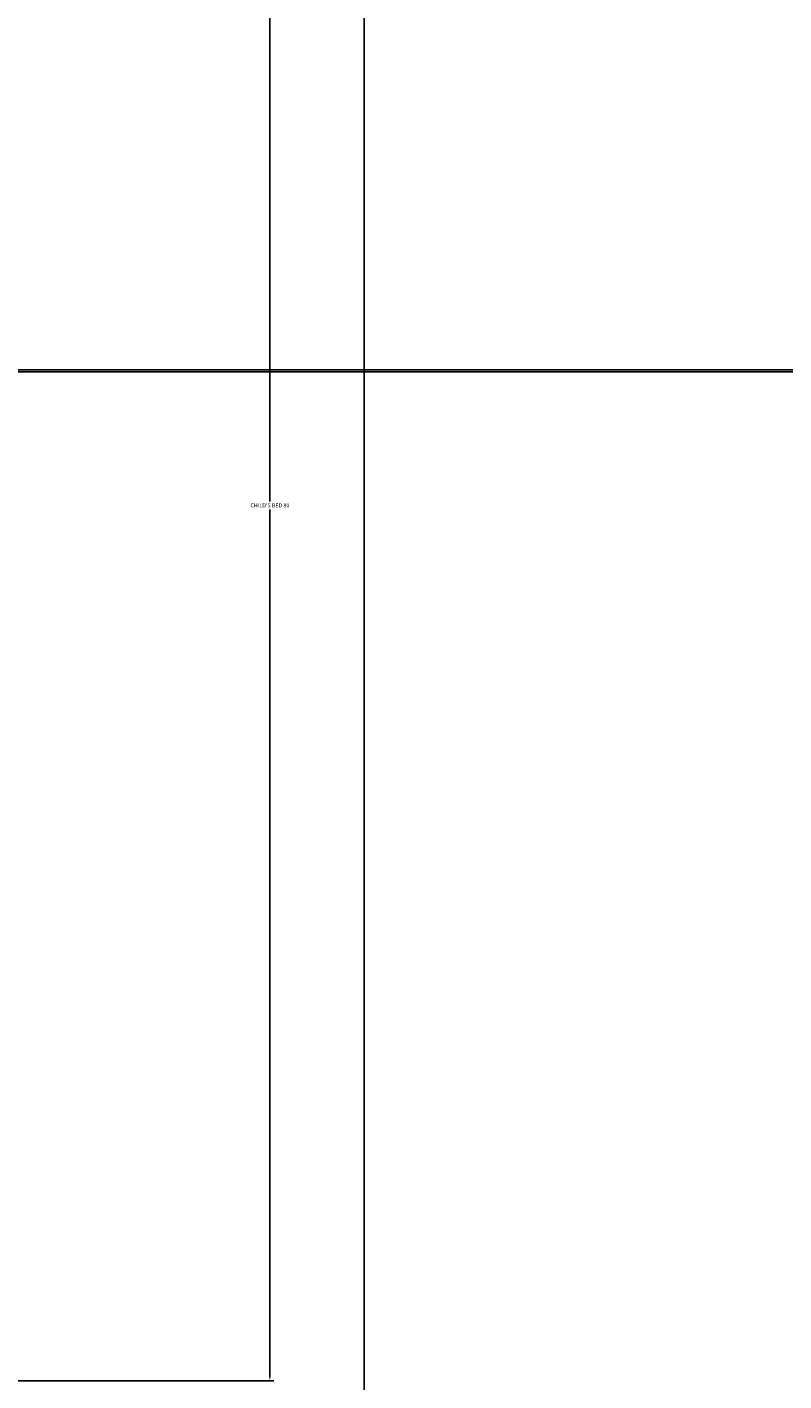
# Model space of a CAD drawing. Units: inches. Extents: x -1517 to -668, y -425 to 52.
# Tile 11 of 13: x -1129 to -1095, y -63 to -1. Entities that reach past the tile are written whole.
import ezdxf

# ---------------------------------------------------------------- set-up
doc = ezdxf.new("R2010")
doc.units = ezdxf.units.IN
doc.header["$MEASUREMENT"] = 0
doc.layers.add('A-ANNO-DIMS', color=2, linetype='Continuous', lineweight=18)
doc.styles.get("Standard").update_dxf_attribs({"font": 'arial.ttf'})
doc.dimstyles.get("Standard").update_dxf_attribs({"dimtxt": 0.18, "dimasz": 0.18, "dimexe": 0.18, "dimexo": 0.0625, "dimgap": 0.09, "dimtad": 0, "dimtih": 1, "dimtoh": 1, "dimdec": 4, "dimzin": 0, "dimdsep": 46, "dimlunit": 4, "dimtxsty": 'Standard', "dimcen": 0.09, "dimadec": 0, "dimazin": 0, "dimtfac": 1, "dimtdec": 4, "dimtofl": 0, "dimtmove": 0, "dimatfit": 3, "dimfxl": 1, "dimtolj": 1, "dimtzin": 0, "dimarcsym": 0})

# ---------------------------------------------------------------- blocks, each defined once
blk = doc.blocks.new('*D36')
at = {"layer": 'A-ANNO-DIMS', "color": 0, "lineweight": -2, "transparency": 16777216}
for p, q in [((-1130.311, 17.63), (-1118.156, 17.63)), ((-1118.336, 17.45), (-1118.336, -22.314)), ((-1118.336, -62.443), (-1118.336, -22.68)), ((-1130.311, -62.623), (-1118.156, -62.623))]:
    blk.add_line(p, q, dxfattribs=at)
at = {"layer": 'A-ANNO-DIMS', "color": 0, "transparency": 16777216}
for points in [[(-1118.366, 17.45), (-1118.306, 17.45), (-1118.336, 17.63)], [(-1118.366, -62.443), (-1118.306, -62.443), (-1118.336, -62.623)]]:
    blk.add_solid(points, dxfattribs=at)
at = {"layer": 'Defpoints', "color": 0, "transparency": 16777216}
for p in [(-1130.374, 17.63), (-1118.336, 17.63), (-1130.374, -62.623)]:
    blk.add_point(p, dxfattribs=at)
at = {"layer": 'A-ANNO-DIMS', "color": 0, "transparency": 16777216, "insert": (-1118.336, -22.497), "char_height": 0.18, "attachment_point": 5}
blk.add_mtext("\\A1;CHILD'S BED 80", dxfattribs=at)
blk = doc.blocks.new('*D53')
at = {"layer": 'A-ANNO-DIMS', "color": 0, "lineweight": -2, "transparency": 16777216}
for p, q in [((-1242.504, -153.307), (-1242.504, 52.11)), ((-1242.324, 51.93), (-1128.794, 51.93)), ((-1014.684, 51.93), (-1128.213, 51.93)), ((-1014.504, -150.307), (-1014.504, 52.11))]:
    blk.add_line(p, q, dxfattribs=at)
at = {"layer": 'A-ANNO-DIMS', "color": 0, "transparency": 16777216}
for points in [[(-1242.324, 51.96), (-1242.324, 51.9), (-1242.504, 51.93)], [(-1014.684, 51.96), (-1014.684, 51.9), (-1014.504, 51.93)]]:
    blk.add_solid(points, dxfattribs=at)
at = {"layer": 'Defpoints', "color": 0, "transparency": 16777216}
for p in [(-1014.504, 51.93), (-1014.504, -150.37), (-1242.504, -153.37)]:
    blk.add_point(p, dxfattribs=at)
at = {"layer": 'A-ANNO-DIMS', "color": 0, "transparency": 16777216, "insert": (-1128.504, 51.93), "char_height": 0.18, "attachment_point": 5}
blk.add_mtext('\\A1;228', dxfattribs=at)
blk = doc.blocks.new('*D57')
at = {"layer": 'A-ANNO-DIMS', "color": 0, "lineweight": -2, "transparency": 16777216}
for p, q in [((-1114.018, -282.307), (-1114.018, 52.11)), ((-1113.838, 51.93), (-1090.241, 51.93)), ((-1066.198, 51.93), (-1089.796, 51.93)), ((-1066.018, -282.307), (-1066.018, 52.11))]:
    blk.add_line(p, q, dxfattribs=at)
at = {"layer": 'A-ANNO-DIMS', "color": 0, "transparency": 16777216}
for points in [[(-1113.838, 51.96), (-1113.838, 51.9), (-1114.018, 51.93)], [(-1066.198, 51.96), (-1066.198, 51.9), (-1066.018, 51.93)]]:
    blk.add_solid(points, dxfattribs=at)
at = {"layer": 'Defpoints', "color": 0, "transparency": 16777216}
for p in [(-1066.018, 51.93), (-1114.018, -282.37), (-1066.018, -282.37)]:
    blk.add_point(p, dxfattribs=at)
at = {"layer": 'A-ANNO-DIMS', "color": 0, "transparency": 16777216, "insert": (-1090.018, 51.93), "char_height": 0.18, "attachment_point": 5}
blk.add_mtext('\\A1;48', dxfattribs=at)
blk = doc.blocks.new('*D65')
at = {"layer": 'A-ANNO-DIMS', "color": 0, "lineweight": -2, "transparency": 16777216}
for p, q in [((-1138.018, -282.307), (-1138.018, 52.11)), ((-1137.838, 51.93), (-1126.238, 51.93)), ((-1114.198, 51.93), (-1125.798, 51.93)), ((-1114.018, -282.307), (-1114.018, 52.11))]:
    blk.add_line(p, q, dxfattribs=at)
at = {"layer": 'A-ANNO-DIMS', "color": 0, "transparency": 16777216}
for points in [[(-1137.838, 51.96), (-1137.838, 51.9), (-1138.018, 51.93)], [(-1114.198, 51.96), (-1114.198, 51.9), (-1114.018, 51.93)]]:
    blk.add_solid(points, dxfattribs=at)
at = {"layer": 'Defpoints', "color": 0, "transparency": 16777216}
for p in [(-1114.018, 51.93), (-1138.018, -282.37), (-1114.018, -282.37)]:
    blk.add_point(p, dxfattribs=at)
at = {"layer": 'A-ANNO-DIMS', "color": 0, "transparency": 16777216, "insert": (-1126.018, 51.93), "char_height": 0.18, "attachment_point": 5}
blk.add_mtext('\\A1;24', dxfattribs=at)
blk = doc.blocks.new('*D72')
at = {"layer": 'A-ANNO-DIMS', "color": 0, "lineweight": -2, "transparency": 16777216}
for p, q in [((-1285.841, -16.282), (-980.024, -16.282)), ((-980.204, -16.462), (-980.204, -59.144)), ((-980.204, -102.19), (-980.204, -59.508)), ((-1285.841, -102.37), (-980.024, -102.37))]:
    blk.add_line(p, q, dxfattribs=at)
at = {"layer": 'A-ANNO-DIMS', "color": 0, "transparency": 16777216}
for points in [[(-980.234, -16.462), (-980.174, -16.462), (-980.204, -16.282)], [(-980.234, -102.19), (-980.174, -102.19), (-980.204, -102.37)]]:
    blk.add_solid(points, dxfattribs=at)
at = {"layer": 'Defpoints', "color": 0, "transparency": 16777216}
for p in [(-1285.904, -16.282), (-1285.904, -102.37), (-980.204, -102.37)]:
    blk.add_point(p, dxfattribs=at)
at = {"layer": 'A-ANNO-DIMS', "color": 0, "transparency": 16777216, "insert": (-980.204, -59.326), "char_height": 0.18, "attachment_point": 5}
blk.add_mtext('\\A1;86.09', dxfattribs=at)
blk = doc.blocks.new('*D73')
at = {"layer": 'A-ANNO-DIMS', "color": 0, "lineweight": -2, "transparency": 16777216}
for p, q in [((-1089.366, -16.37), (-1516.984, -16.37)), ((-1516.804, -16.55), (-1516.804, -59.188)), ((-1516.804, -102.19), (-1516.804, -59.552)), ((-1089.366, -102.37), (-1516.984, -102.37))]:
    blk.add_line(p, q, dxfattribs=at)
at = {"layer": 'A-ANNO-DIMS', "color": 0, "transparency": 16777216}
for points in [[(-1516.834, -16.55), (-1516.774, -16.55), (-1516.804, -16.37)], [(-1516.834, -102.19), (-1516.774, -102.19), (-1516.804, -102.37)]]:
    blk.add_solid(points, dxfattribs=at)
at = {"layer": 'Defpoints', "color": 0, "transparency": 16777216}
for p in [(-1089.304, -16.37), (-1516.804, -102.37), (-1089.304, -102.37)]:
    blk.add_point(p, dxfattribs=at)
at = {"layer": 'A-ANNO-DIMS', "color": 0, "transparency": 16777216, "insert": (-1516.804, -59.37), "char_height": 0.18, "attachment_point": 5}
blk.add_mtext('\\A1;86', dxfattribs=at)

msp = doc.modelspace()

# ---------------------------------------------------------------- dimensions: what is measured, and where the dimension line sits
at = {"layer": 'A-ANNO-DIMS'}
for base, p1, p2, picture, middle in [((-1014.5037, 51.93), (-1242.5037, -153.37), (-1014.5037, -150.37), '*D53', (-1128.5037, 51.93)), ((-1114.0183, 51.93), (-1138.0183, -282.37), (-1114.0183, -282.37), '*D65', (-1126.0183, 51.93)), ((-1066.0183, 51.93), (-1114.0183, -282.37), (-1066.0183, -282.37), '*D57', (-1090.0183, 51.93))]:
    dim = msp.add_linear_dim(base=base, p1=p1, p2=p2, dimstyle='Standard', override={"dimdec": 0, "dimlfac": 1, "dimrnd": 0, "dimzin": 0, "dimdsep": 46, "dimlunit": 2}, dxfattribs=at)
    dim.commit()
    dim.dimension.update_dxf_attribs({"geometry": picture, "text_midpoint": middle})
dim = msp.add_linear_dim(base=(-1118.336, 17.63), p1=(-1130.374, -62.6234), p2=(-1130.374, 17.63), angle=90, text="CHILD'S BED <>", dimstyle='Standard', override={"dimdec": 0, "dimlfac": 1, "dimrnd": 0, "dimzin": 0, "dimdsep": 46, "dimlunit": 2}, dxfattribs=at)
dim.commit()
dim.dimension.update_dxf_attribs({"geometry": '*D36', "text_midpoint": (-1118.336, -22.4967)})
for base, p1, p2, override, picture, middle in [((-1516.8037, -102.37), (-1089.3037, -16.37), (-1089.3037, -102.37), {"dimdec": 0, "dimlfac": 1, "dimrnd": 0, "dimzin": 0, "dimdsep": 46, "dimlunit": 2}, '*D73', (-1516.8037, -59.37)), ((-980.2037, -102.37), (-1285.9037, -16.2817), (-1285.9037, -102.37), {"dimdec": 2, "dimlfac": 1, "dimrnd": 0, "dimzin": 0, "dimdsep": 46, "dimlunit": 2}, '*D72', (-980.2037, -59.3258))]:
    dim = msp.add_linear_dim(base=base, p1=p1, p2=p2, angle=90, dimstyle='Standard', override=override, dxfattribs=at)
    dim.commit()
    dim.dimension.update_dxf_attribs({"geometry": picture, "text_midpoint": middle})

doc.saveas('drawing.dxf')
